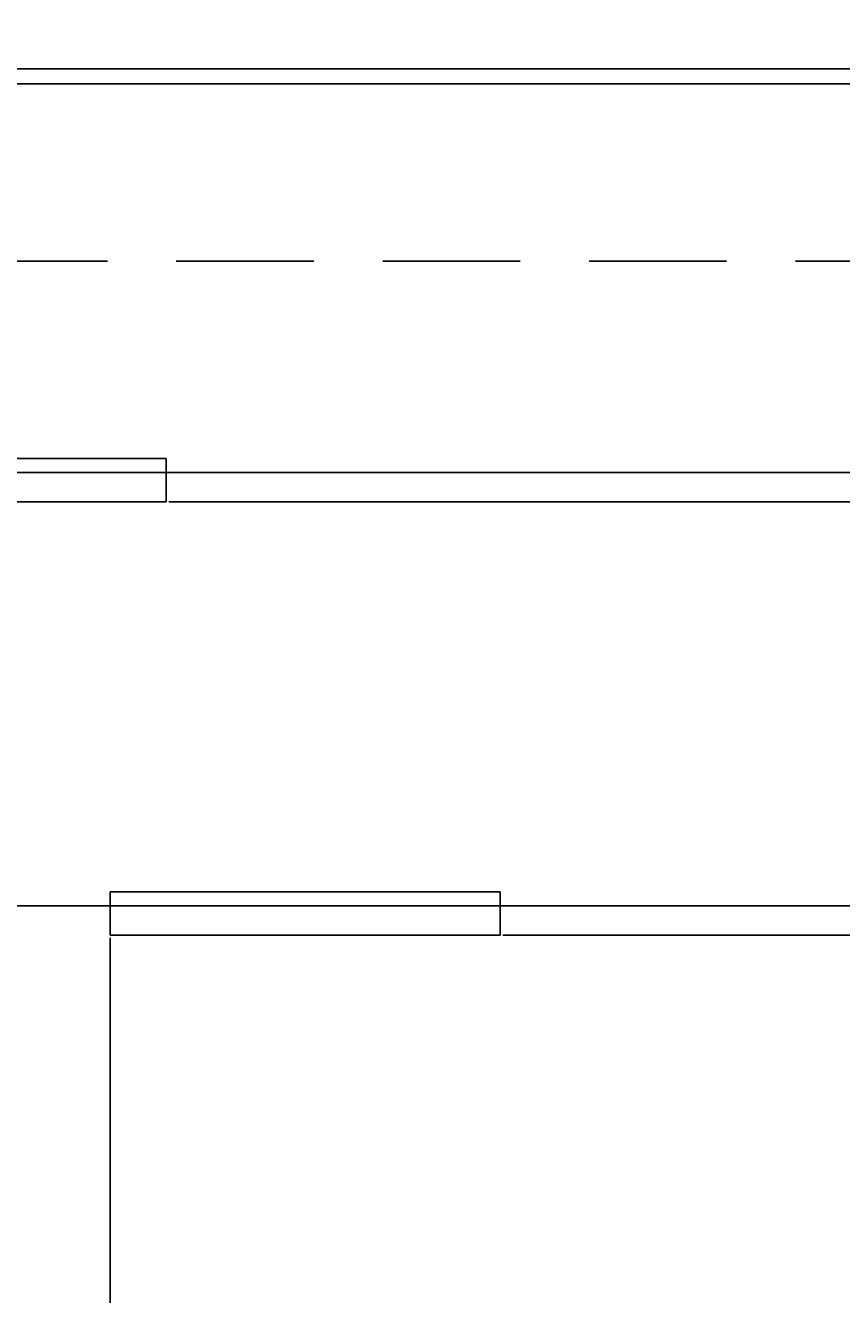
# Model space of a CAD drawing. Units: inches. Extents: x 2812 to 3051, y 1398 to 1659.
# Tile 32 of 65: x 2985 to 3004, y 1438 to 1468. Entities that reach past the tile are written whole.
import ezdxf

# ---------------------------------------------------------------- set-up
doc = ezdxf.new("R2010")
doc.units = ezdxf.units.IN
doc.linetypes.add('HIDDEN2', pattern=[4.7625, 3.175, -1.5875])
for name, color, linetype, lineweight in [('A-ANNO-DIMS', 2, 'Continuous', 18), ('S-CONC-HIDN', 8, 'HIDDEN2', 25), ('S-STEP', 3, 'Continuous', 25)]:
    doc.layers.add(name, color=color, linetype=linetype, lineweight=lineweight)
doc.styles.get("Standard").update_dxf_attribs({"font": 'arial.ttf'})
doc.dimstyles.get("Standard").update_dxf_attribs({"dimtxt": 0.18, "dimasz": 0.18, "dimexe": 0.18, "dimexo": 0.0625, "dimgap": 0.09, "dimtad": 0, "dimtih": 1, "dimtoh": 1, "dimdec": 4, "dimzin": 0, "dimdsep": 46, "dimtxsty": 'Standard', "dimcen": 0.09, "dimadec": 0, "dimazin": 0, "dimtfac": 1, "dimtdec": 4, "dimtofl": 0, "dimtmove": 0, "dimatfit": 3, "dimfxl": 1, "dimtolj": 1, "dimtzin": 0, "dimarcsym": 0})

# ---------------------------------------------------------------- blocks, each defined once
blk = doc.blocks.new('STEP-IRON-1')
for p, q in [((9, 1), (0, 1)), ((0, 1), (0, 0)), ((9, 0), (9, 1)), ((0, 0), (9, 0)), ((0, 0), (5.792, 0)), ((0, 0), (1.139, 0))]:
    blk.add_line(p, q)
blk = doc.blocks.new('STEP-IRON-4')
for p, q in [((9, 1), (0, 1)), ((0, 1), (0, 0)), ((9, 0), (9, 1)), ((0, 0), (9, 0)), ((0, 0), (5.792, 0))]:
    blk.add_line(p, q)
blk = doc.blocks.new('*D47')
at = {"layer": 'A-ANNO-DIMS', "color": 0, "lineweight": -2, "transparency": 16777216}
for p, q in [((2970.385, 1487.973), (2970.385, 1397.505)), ((3006.385, 1487.973), (3006.385, 1397.505)), ((2970.565, 1397.685), (2988.166, 1397.685)), ((3006.205, 1397.685), (2988.604, 1397.685))]:
    blk.add_line(p, q, dxfattribs=at)
at = {"layer": 'A-ANNO-DIMS', "color": 0, "transparency": 16777216}
for points in [[(2970.565, 1397.715), (2970.565, 1397.655), (2970.385, 1397.685)], [(3006.205, 1397.715), (3006.205, 1397.655), (3006.385, 1397.685)]]:
    blk.add_solid(points, dxfattribs=at)
at = {"layer": 'Defpoints', "color": 0, "transparency": 16777216}
for p in [(2970.385, 1488.035), (3006.385, 1488.035), (3006.385, 1397.685)]:
    blk.add_point(p, dxfattribs=at)
at = {"layer": 'A-ANNO-DIMS', "color": 0, "transparency": 16777216, "insert": (2988.385, 1397.685), "char_height": 0.18, "attachment_point": 5}
blk.add_mtext('\\A1;36', dxfattribs=at)
blk = doc.blocks.new('*D66')
at = {"layer": 'A-ANNO-DIMS', "color": 0, "lineweight": -2, "transparency": 16777216}
for p, q in [((2914.018, 1447.426), (3051.178, 1447.426)), ((3050.998, 1447.246), (3050.998, 1442.608)), ((3050.998, 1437.606), (3050.998, 1442.245)), ((2920.62, 1437.426), (3051.178, 1437.426))]:
    blk.add_line(p, q, dxfattribs=at)
at = {"layer": 'A-ANNO-DIMS', "color": 0, "transparency": 16777216}
for points in [[(3050.968, 1447.246), (3051.028, 1447.246), (3050.998, 1447.426)], [(3050.968, 1437.606), (3051.028, 1437.606), (3050.998, 1437.426)]]:
    blk.add_solid(points, dxfattribs=at)
at = {"layer": 'Defpoints', "color": 0, "transparency": 16777216}
for p in [(2913.955, 1447.426), (3050.998, 1447.426), (2920.558, 1437.426)]:
    blk.add_point(p, dxfattribs=at)
at = {"layer": 'A-ANNO-DIMS', "color": 0, "transparency": 16777216, "insert": (3050.998, 1442.426), "char_height": 0.18, "attachment_point": 5}
blk.add_mtext('\\A1;10', dxfattribs=at)
blk = doc.blocks.new('*D67')
at = {"layer": 'A-ANNO-DIMS', "color": 0, "lineweight": -2, "transparency": 16777216}
for p, q in [((2906.065, 1457.426), (3051.178, 1457.426)), ((3050.998, 1457.246), (3050.998, 1452.608)), ((3050.998, 1447.606), (3050.998, 1452.245)), ((2914.018, 1447.426), (3051.178, 1447.426))]:
    blk.add_line(p, q, dxfattribs=at)
at = {"layer": 'A-ANNO-DIMS', "color": 0, "transparency": 16777216}
for points in [[(3050.968, 1457.246), (3051.028, 1457.246), (3050.998, 1457.426)], [(3050.968, 1447.606), (3051.028, 1447.606), (3050.998, 1447.426)]]:
    blk.add_solid(points, dxfattribs=at)
at = {"layer": 'Defpoints', "color": 0, "transparency": 16777216}
for p in [(2906.002, 1457.426), (3050.998, 1457.426), (2913.955, 1447.426)]:
    blk.add_point(p, dxfattribs=at)
at = {"layer": 'A-ANNO-DIMS', "color": 0, "transparency": 16777216, "insert": (3050.998, 1452.426), "char_height": 0.18, "attachment_point": 5}
blk.add_mtext('\\A1;10', dxfattribs=at)
blk = doc.blocks.new('*D68')
at = {"layer": 'A-ANNO-DIMS', "color": 0, "lineweight": -2, "transparency": 16777216}
for p, q in [((2898.12, 1466.402), (3051.178, 1466.402)), ((3050.998, 1466.222), (3050.998, 1462.096)), ((3050.998, 1457.606), (3050.998, 1461.733)), ((2906.065, 1457.426), (3051.178, 1457.426))]:
    blk.add_line(p, q, dxfattribs=at)
at = {"layer": 'A-ANNO-DIMS', "color": 0, "transparency": 16777216}
for points in [[(3050.968, 1466.222), (3051.028, 1466.222), (3050.998, 1466.402)], [(3050.968, 1457.606), (3051.028, 1457.606), (3050.998, 1457.426)]]:
    blk.add_solid(points, dxfattribs=at)
at = {"layer": 'Defpoints', "color": 0, "transparency": 16777216}
for p in [(2898.058, 1466.402), (3050.998, 1466.402), (2906.002, 1457.426)]:
    blk.add_point(p, dxfattribs=at)
at = {"layer": 'A-ANNO-DIMS', "color": 0, "transparency": 16777216, "insert": (3050.998, 1461.914), "char_height": 0.18, "attachment_point": 5}
blk.add_mtext('\\A1;8.976', dxfattribs=at)
blk = doc.blocks.new('*D72')
at = {"layer": 'A-ANNO-DIMS', "color": 0, "lineweight": -2, "transparency": 16777216}
for p, q in [((2979.248, 1456.685), (2979.248, 1397.505)), ((2986.956, 1446.685), (2986.956, 1397.505)), ((2979.428, 1397.685), (2982.709, 1397.685)), ((2986.776, 1397.685), (2983.495, 1397.685))]:
    blk.add_line(p, q, dxfattribs=at)
at = {"layer": 'A-ANNO-DIMS', "color": 0, "transparency": 16777216}
for points in [[(2979.428, 1397.715), (2979.428, 1397.655), (2979.248, 1397.685)], [(2986.776, 1397.715), (2986.776, 1397.655), (2986.956, 1397.685)]]:
    blk.add_solid(points, dxfattribs=at)
at = {"layer": 'Defpoints', "color": 0, "transparency": 16777216}
for p in [(2979.248, 1456.747), (2986.956, 1446.747), (2986.956, 1397.685)]:
    blk.add_point(p, dxfattribs=at)
at = {"layer": 'A-ANNO-DIMS', "color": 0, "transparency": 16777216, "insert": (2983.102, 1397.685), "char_height": 0.18, "attachment_point": 5}
blk.add_mtext('\\A1;7.708', dxfattribs=at)
blk = doc.blocks.new('*D73')
at = {"layer": 'A-ANNO-DIMS', "color": 0, "lineweight": -2, "transparency": 16777216}
for p, q in [((2986.956, 1446.685), (2986.956, 1397.505)), ((2994.221, 1436.685), (2994.221, 1397.505)), ((2987.136, 1397.685), (2990.195, 1397.685)), ((2994.041, 1397.685), (2990.982, 1397.685))]:
    blk.add_line(p, q, dxfattribs=at)
at = {"layer": 'A-ANNO-DIMS', "color": 0, "transparency": 16777216}
for points in [[(2987.136, 1397.715), (2987.136, 1397.655), (2986.956, 1397.685)], [(2994.041, 1397.715), (2994.041, 1397.655), (2994.221, 1397.685)]]:
    blk.add_solid(points, dxfattribs=at)
at = {"layer": 'Defpoints', "color": 0, "transparency": 16777216}
for p in [(2986.956, 1446.747), (2994.221, 1436.747), (2994.221, 1397.685)]:
    blk.add_point(p, dxfattribs=at)
at = {"layer": 'A-ANNO-DIMS', "color": 0, "transparency": 16777216, "insert": (2990.589, 1397.685), "char_height": 0.18, "attachment_point": 5}
blk.add_mtext('\\A1;7.265', dxfattribs=at)
blk = doc.blocks.new('*D80')
at = {"layer": 'A-ANNO-DIMS', "color": 0, "lineweight": -2, "transparency": 16777216}
for p, q in [((2996.018, 1446.747), (3051.178, 1446.747)), ((3050.998, 1446.567), (3050.998, 1441.929)), ((3050.998, 1436.927), (3050.998, 1441.565)), ((3003.284, 1436.747), (3051.178, 1436.747))]:
    blk.add_line(p, q, dxfattribs=at)
at = {"layer": 'A-ANNO-DIMS', "color": 0, "transparency": 16777216}
for points in [[(3050.968, 1446.567), (3051.028, 1446.567), (3050.998, 1446.747)], [(3050.968, 1436.927), (3051.028, 1436.927), (3050.998, 1436.747)]]:
    blk.add_solid(points, dxfattribs=at)
at = {"layer": 'Defpoints', "color": 0, "transparency": 16777216}
for p in [(2995.956, 1446.747), (3050.998, 1446.747), (3003.221, 1436.747)]:
    blk.add_point(p, dxfattribs=at)
at = {"layer": 'A-ANNO-DIMS', "color": 0, "transparency": 16777216, "insert": (3050.998, 1441.747), "char_height": 0.18, "attachment_point": 5}
blk.add_mtext('\\A1;10', dxfattribs=at)
blk = doc.blocks.new('*D81')
at = {"layer": 'A-ANNO-DIMS', "color": 0, "lineweight": -2, "transparency": 16777216}
for p, q in [((2988.31, 1456.747), (3051.178, 1456.747)), ((3050.998, 1456.567), (3050.998, 1451.929)), ((3050.998, 1446.927), (3050.998, 1451.565)), ((2996.018, 1446.747), (3051.178, 1446.747))]:
    blk.add_line(p, q, dxfattribs=at)
at = {"layer": 'A-ANNO-DIMS', "color": 0, "transparency": 16777216}
for points in [[(3050.968, 1456.567), (3051.028, 1456.567), (3050.998, 1456.747)], [(3050.968, 1446.927), (3051.028, 1446.927), (3050.998, 1446.747)]]:
    blk.add_solid(points, dxfattribs=at)
at = {"layer": 'Defpoints', "color": 0, "transparency": 16777216}
for p in [(2988.248, 1456.747), (3050.998, 1456.747), (2995.956, 1446.747)]:
    blk.add_point(p, dxfattribs=at)
at = {"layer": 'A-ANNO-DIMS', "color": 0, "transparency": 16777216, "insert": (3050.998, 1451.747), "char_height": 0.18, "attachment_point": 5}
blk.add_mtext('\\A1;10', dxfattribs=at)
blk = doc.blocks.new('*D82')
at = {"layer": 'A-ANNO-DIMS', "color": 0, "lineweight": -2, "transparency": 16777216}
for p, q in [((2978.018, 1466.747), (3051.178, 1466.747)), ((3050.998, 1466.567), (3050.998, 1461.929)), ((3050.998, 1456.927), (3050.998, 1461.565)), ((2988.31, 1456.747), (3051.178, 1456.747))]:
    blk.add_line(p, q, dxfattribs=at)
at = {"layer": 'A-ANNO-DIMS', "color": 0, "transparency": 16777216}
for points in [[(3050.968, 1466.567), (3051.028, 1466.567), (3050.998, 1466.747)], [(3050.968, 1456.927), (3051.028, 1456.927), (3050.998, 1456.747)]]:
    blk.add_solid(points, dxfattribs=at)
at = {"layer": 'Defpoints', "color": 0, "transparency": 16777216}
for p in [(2977.956, 1466.747), (3050.998, 1466.747), (2988.248, 1456.747)]:
    blk.add_point(p, dxfattribs=at)
at = {"layer": 'A-ANNO-DIMS', "color": 0, "transparency": 16777216, "insert": (3050.998, 1461.747), "char_height": 0.18, "attachment_point": 5}
blk.add_mtext('\\A1;10', dxfattribs=at)

msp = doc.modelspace()

# ---------------------------------------------------------------- linework, layer by layer
at = {"layer": 'S-CONC-HIDN'}
msp.add_line((3029.7562, 1462.3026), (2835.3849, 1462.3026), dxfattribs=at)

# ---------------------------------------------------------------- block references
at = {"layer": 'S-STEP'}
for name, p in [('STEP-IRON-4', (2979.248, 1456.747)), ('STEP-IRON-1', (2986.956, 1446.747))]:
    msp.add_blockref(name, p, dxfattribs=at)

# ---------------------------------------------------------------- dimensions: what is measured, and where the dimension line sits
at = {"layer": 'A-ANNO-DIMS'}
for base, p1, p2, override, picture, middle in [((3006.3849, 1397.6854), (2970.3849, 1488.0354), (3006.3849, 1488.0354), {"dimdec": 0, "dimlfac": 1, "dimrnd": 0, "dimzin": 0, "dimdsep": 46, "dimlunit": 2}, '*D47', (2988.3849, 1397.6854)), ((2986.9558, 1397.6854), (2979.2478, 1456.7474), (2986.9558, 1446.7474), {"dimdec": 3, "dimlfac": 1, "dimrnd": 0, "dimzin": 0, "dimdsep": 46, "dimlunit": 2}, '*D72', (2983.1018, 1397.6854)), ((2994.22128, 1397.6854), (2986.95585, 1446.74738), (2994.22128, 1436.74738), {"dimdec": 3, "dimlfac": 1, "dimrnd": 0, "dimzin": 0, "dimdsep": 46, "dimlunit": 2}, '*D73', (2990.58856, 1397.6854))]:
    dim = msp.add_linear_dim(base=base, p1=p1, p2=p2, dimstyle='Standard', override=override, dxfattribs=at)
    dim.commit()
    dim.dimension.update_dxf_attribs({"geometry": picture, "text_midpoint": middle})
for base, p1, p2, override, picture, middle in [((3050.998, 1466.7474), (2988.2478, 1456.7474), (2977.9558, 1466.7474), {"dimdec": 0, "dimlfac": 1, "dimrnd": 0, "dimzin": 0, "dimdsep": 46, "dimlunit": 2}, '*D82', (3050.998, 1461.7474)), ((3050.998, 1466.4024), (2906.0021, 1457.4265), (2898.0577, 1466.4024), {"dimdec": 3, "dimlfac": 1, "dimrnd": 0, "dimzin": 0, "dimdsep": 46, "dimlunit": 2}, '*D68', (3050.998, 1461.9144)), ((3050.998, 1457.4265), (2913.9551, 1447.4265), (2906.0021, 1457.4265), {"dimdec": 0, "dimlfac": 1, "dimrnd": 0, "dimzin": 0, "dimdsep": 46, "dimlunit": 2}, '*D67', (3050.998, 1452.4265)), ((3050.998, 1456.7474), (2995.9558, 1446.7474), (2988.2478, 1456.7474), {"dimdec": 0, "dimlfac": 1, "dimrnd": 0, "dimzin": 0, "dimdsep": 46, "dimlunit": 2}, '*D81', (3050.998, 1451.7474)), ((3050.998, 1447.4265), (2920.5577, 1437.4265), (2913.9551, 1447.4265), {"dimdec": 0, "dimlfac": 1, "dimrnd": 0, "dimzin": 0, "dimdsep": 46, "dimlunit": 2}, '*D66', (3050.998, 1442.4265)), ((3050.998, 1446.7474), (3003.2213, 1436.7474), (2995.9558, 1446.7474), {"dimdec": 0, "dimlfac": 1, "dimrnd": 0, "dimzin": 0, "dimdsep": 46, "dimlunit": 2}, '*D80', (3050.998, 1441.7474))]:
    dim = msp.add_linear_dim(base=base, p1=p1, p2=p2, angle=90, dimstyle='Standard', override=override, dxfattribs=at)
    dim.commit()
    dim.dimension.update_dxf_attribs({"geometry": picture, "text_midpoint": middle})

doc.saveas('drawing.dxf')
